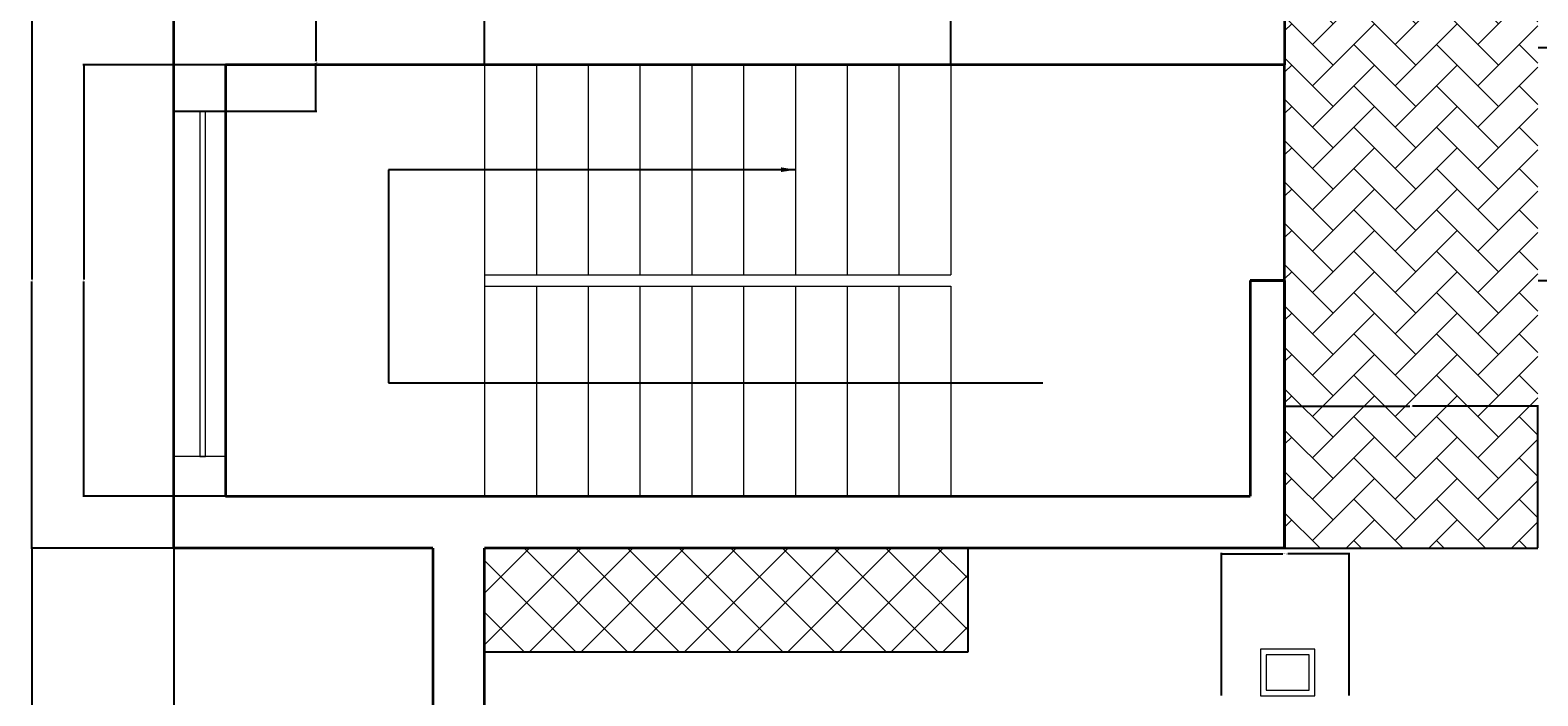
# Model space of a CAD drawing. Units: inches. Extents: x 1315 to 1802, y 1702 to 2202.
# Tile 2 of 4: x 1315 to 1577, y 1906 to 2021. Entities that reach past the tile are written whole.
import ezdxf

# ---------------------------------------------------------------- set-up
doc = ezdxf.new("R2010")
doc.units = ezdxf.units.IN
for name, color, linetype, lineweight in [('A-ANNO-DIMS', 2, 'Continuous', 18), ('A-CASE', 7, 'Continuous', 25), ('A-CASE-PATT', 246, 'Continuous', 13), ('A-FLOR', 7, 'Continuous', 25), ('A-FLOR-PATT', 254, 'Continuous', 13), ('A-FLOR-STRS', 7, 'Continuous', 18), ('A-FURN', 8, 'Continuous', 18), ('A-GLAZ', 4, 'Continuous', 18), ('A-WALL', 7, 'Continuous', 35)]:
    doc.layers.add(name, color=color, linetype=linetype, lineweight=lineweight)
doc.styles.get("Standard").update_dxf_attribs({"font": 'times.ttf'})
doc.dimstyles.new('ISO-25', dxfattribs={"dimtxt": 2.5, "dimasz": 2.5, "dimexe": 1.25, "dimexo": 0.625, "dimtad": 1, "dimdsep": 46, "dimlunit": 3, "dimtxsty": 'Standard', "dimcen": 5, "dimadec": 0, "dimazin": 0, "dimtfac": 1, "dimtmove": 0, "dimatfit": 3, "dimfxl": 1, "dimarcsym": 0})
doc.dimstyles.get("Standard").update_dxf_attribs({"dimtxt": 0.18, "dimasz": 0.18, "dimexe": 0.18, "dimexo": 0.0625, "dimgap": 0.09, "dimtad": 0, "dimtih": 1, "dimtoh": 1, "dimdec": 4, "dimzin": 0, "dimdsep": 46, "dimtxsty": 'Standard', "dimcen": 0.09, "dimadec": 0, "dimazin": 0, "dimtfac": 1, "dimtdec": 4, "dimtofl": 0, "dimtmove": 0, "dimatfit": 3, "dimfxl": 1, "dimtolj": 1, "dimtzin": 0, "dimarcsym": 0})

# ---------------------------------------------------------------- blocks, each defined once
blk = doc.blocks.new('SEFVFT')
for p, q in [((1768.59, 1985.26), (1777.59, 1985.26)), ((1768.59, 1925.26), (1768.59, 1985.26)), ((1768.59, 1985.26), (1773.09, 1985.26)), ((1773.09, 1985.26), (1773.09, 1925.26)), ((1774.09, 1925.26), (1774.09, 1985.26)), ((1777.59, 1985.26), (1777.59, 1925.26)), ((1777.59, 1925.26), (1768.59, 1925.26)), ((1773.09, 1925.26), (1774.09, 1925.26))]:
    blk.add_line(p, q)
blk = doc.blocks.new('CHAIR-DINING-END')
for points in [[(0, 0), (9.48, 0), (9.48, 8.13), (0, 8.13)], [(1, 1), (8.48, 1), (8.48, 7.13), (1, 7.13)]]:
    blk.add_lwpolyline(points, close=True)
blk = doc.blocks.new('*D28')
at = {"layer": 'A-ANNO-DIMS', "color": 0, "lineweight": -2, "transparency": 16777216}
for p, q in [((1339.59, 1931.18), (1339.59, 1702.41)), ((1777.59, 1763.18), (1777.59, 1702.41)), ((1339.77, 1702.59), (1558.31, 1702.59)), ((1777.41, 1702.59), (1558.87, 1702.59))]:
    blk.add_line(p, q, dxfattribs=at)
at = {"layer": 'A-ANNO-DIMS', "color": 0, "transparency": 16777216}
for points in [[(1339.77, 1702.62), (1339.77, 1702.56), (1339.59, 1702.59)], [(1777.41, 1702.62), (1777.41, 1702.56), (1777.59, 1702.59)]]:
    blk.add_solid(points, dxfattribs=at)
at = {"layer": 'Defpoints', "color": 0, "transparency": 16777216}
for p in [(1339.59, 1931.24), (1777.59, 1763.24), (1777.59, 1702.59)]:
    blk.add_point(p, dxfattribs=at)
at = {"layer": 'A-ANNO-DIMS', "color": 0, "transparency": 16777216, "insert": (1558.59, 1702.59), "char_height": 0.18, "attachment_point": 5}
blk.add_mtext('\\A1;438', dxfattribs=at)
blk = doc.blocks.new('*D37')
at = {"layer": 'A-ANNO-DIMS', "color": 0, "lineweight": -2, "transparency": 16777216}
for p, q in [((1339.53, 2024.24), (1314.76, 2024.24)), ((1314.94, 2024.06), (1314.94, 1977.92)), ((1314.94, 1931.42), (1314.94, 1977.56)), ((1339.53, 1931.24), (1314.76, 1931.24))]:
    blk.add_line(p, q, dxfattribs=at)
at = {"layer": 'A-ANNO-DIMS', "color": 0, "transparency": 16777216}
for points in [[(1314.91, 2024.06), (1314.97, 2024.06), (1314.94, 2024.24)], [(1314.91, 1931.42), (1314.97, 1931.42), (1314.94, 1931.24)]]:
    blk.add_solid(points, dxfattribs=at)
at = {"layer": 'Defpoints', "color": 0, "transparency": 16777216}
for p in [(1339.59, 2024.24), (1314.94, 1931.24), (1339.59, 1931.24)]:
    blk.add_point(p, dxfattribs=at)
at = {"layer": 'A-ANNO-DIMS', "color": 0, "transparency": 16777216, "insert": (1314.94, 1977.74), "char_height": 0.18, "attachment_point": 5}
blk.add_mtext('\\A1;93', dxfattribs=at)
blk = doc.blocks.new('*D38')
at = {"layer": 'A-ANNO-DIMS', "color": 0, "lineweight": -2, "transparency": 16777216}
for p, q in [((1339.65, 2024.24), (1364.42, 2024.24)), ((1364.24, 2024.06), (1364.24, 2015.88)), ((1364.24, 2007.33), (1364.24, 2015.51)), ((1339.65, 2007.15), (1364.42, 2007.15))]:
    blk.add_line(p, q, dxfattribs=at)
at = {"layer": 'A-ANNO-DIMS', "color": 0, "transparency": 16777216}
for points in [[(1364.21, 2024.06), (1364.27, 2024.06), (1364.24, 2024.24)], [(1364.21, 2007.33), (1364.27, 2007.33), (1364.24, 2007.15)]]:
    blk.add_solid(points, dxfattribs=at)
at = {"layer": 'Defpoints', "color": 0, "transparency": 16777216}
for p in [(1339.59, 2024.24), (1339.59, 2007.15), (1364.24, 2007.15)]:
    blk.add_point(p, dxfattribs=at)
at = {"layer": 'A-ANNO-DIMS', "color": 0, "transparency": 16777216, "insert": (1364.24, 2015.69), "char_height": 0.18, "attachment_point": 5}
blk.add_mtext('\\A1;17.095', dxfattribs=at)
blk = doc.blocks.new('*D39')
at = {"layer": 'A-ANNO-DIMS', "color": 0, "lineweight": -2, "transparency": 16777216}
for p, q in [((1384.53, 1931.24), (1314.76, 1931.24)), ((1314.94, 1931.06), (1314.94, 1901.56)), ((1314.94, 1871.7), (1314.94, 1901.2)), ((1384.53, 1871.52), (1314.76, 1871.52))]:
    blk.add_line(p, q, dxfattribs=at)
at = {"layer": 'A-ANNO-DIMS', "color": 0, "transparency": 16777216}
for points in [[(1314.91, 1931.06), (1314.97, 1931.06), (1314.94, 1931.24)], [(1314.91, 1871.7), (1314.97, 1871.7), (1314.94, 1871.52)]]:
    blk.add_solid(points, dxfattribs=at)
at = {"layer": 'Defpoints', "color": 0, "transparency": 16777216}
for p in [(1384.59, 1931.24), (1314.94, 1871.52), (1384.59, 1871.52)]:
    blk.add_point(p, dxfattribs=at)
at = {"layer": 'A-ANNO-DIMS', "color": 0, "transparency": 16777216, "insert": (1314.94, 1901.38), "char_height": 0.18, "attachment_point": 5}
blk.add_mtext('\\A1;59.72', dxfattribs=at)
blk = doc.blocks.new('*D49')
at = {"layer": 'A-ANNO-DIMS', "color": 0, "lineweight": -2, "transparency": 16777216}
for p, q in [((1532.59, 1931.3), (1532.59, 1956.07)), ((1532.77, 1955.89), (1554.37, 1955.89)), ((1576.41, 1955.89), (1554.81, 1955.89)), ((1576.59, 1931.3), (1576.59, 1956.07))]:
    blk.add_line(p, q, dxfattribs=at)
at = {"layer": 'A-ANNO-DIMS', "color": 0, "transparency": 16777216}
for points in [[(1532.77, 1955.92), (1532.77, 1955.86), (1532.59, 1955.89)], [(1576.41, 1955.92), (1576.41, 1955.86), (1576.59, 1955.89)]]:
    blk.add_solid(points, dxfattribs=at)
at = {"layer": 'Defpoints', "color": 0, "transparency": 16777216}
for p in [(1576.59, 1955.89), (1532.59, 1931.24), (1576.59, 1931.24)]:
    blk.add_point(p, dxfattribs=at)
at = {"layer": 'A-ANNO-DIMS', "color": 0, "transparency": 16777216, "insert": (1554.59, 1955.89), "char_height": 0.18, "attachment_point": 5}
blk.add_mtext('\\A1;44', dxfattribs=at)
blk = doc.blocks.new('*D50')
at = {"layer": 'A-ANNO-DIMS', "color": 0, "lineweight": -2, "transparency": 16777216}
for p, q in [((1393.59, 2015.3), (1393.59, 2040.07)), ((1393.77, 2039.89), (1433.89, 2039.89)), ((1474.41, 2039.89), (1434.29, 2039.89)), ((1474.59, 2015.3), (1474.59, 2040.07))]:
    blk.add_line(p, q, dxfattribs=at)
at = {"layer": 'A-ANNO-DIMS', "color": 0, "transparency": 16777216}
for points in [[(1393.77, 2039.92), (1393.77, 2039.86), (1393.59, 2039.89)], [(1474.41, 2039.92), (1474.41, 2039.86), (1474.59, 2039.89)]]:
    blk.add_solid(points, dxfattribs=at)
at = {"layer": 'Defpoints', "color": 0, "transparency": 16777216}
for p in [(1474.59, 2039.89), (1393.59, 2015.24), (1474.59, 2015.24)]:
    blk.add_point(p, dxfattribs=at)
at = {"layer": 'A-ANNO-DIMS', "color": 0, "transparency": 16777216, "insert": (1434.09, 2039.89), "char_height": 0.18, "attachment_point": 5}
blk.add_mtext('\\A1;81', dxfattribs=at)
blk = doc.blocks.new('*D51')
at = {"layer": 'A-ANNO-DIMS', "color": 0, "lineweight": -2, "transparency": 16777216}
for p, q in [((1348.53, 2015.24), (1323.76, 2015.24)), ((1323.94, 2015.06), (1323.94, 1977.92)), ((1323.94, 1940.42), (1323.94, 1977.56)), ((1348.53, 1940.24), (1323.76, 1940.24))]:
    blk.add_line(p, q, dxfattribs=at)
at = {"layer": 'A-ANNO-DIMS', "color": 0, "transparency": 16777216}
for points in [[(1323.91, 2015.06), (1323.97, 2015.06), (1323.94, 2015.24)], [(1323.91, 1940.42), (1323.97, 1940.42), (1323.94, 1940.24)]]:
    blk.add_solid(points, dxfattribs=at)
at = {"layer": 'Defpoints', "color": 0, "transparency": 16777216}
for p in [(1323.94, 2015.24), (1348.59, 2015.24), (1348.59, 1940.24)]:
    blk.add_point(p, dxfattribs=at)
at = {"layer": 'A-ANNO-DIMS', "color": 0, "transparency": 16777216, "insert": (1323.94, 1977.74), "char_height": 0.18, "attachment_point": 5}
blk.add_mtext('\\A1;75', dxfattribs=at)
blk = doc.blocks.new('*D52')
at = {"layer": 'A-ANNO-DIMS', "color": 0, "lineweight": -2, "transparency": 16777216}
for p, q in [((1576.65, 2018.24), (1601.42, 2018.24)), ((1601.24, 2018.06), (1601.24, 1998.17)), ((1601.24, 1977.92), (1601.24, 1997.81)), ((1576.65, 1977.74), (1601.42, 1977.74))]:
    blk.add_line(p, q, dxfattribs=at)
at = {"layer": 'A-ANNO-DIMS', "color": 0, "transparency": 16777216}
for points in [[(1601.21, 2018.06), (1601.27, 2018.06), (1601.24, 2018.24)], [(1601.21, 1977.92), (1601.27, 1977.92), (1601.24, 1977.74)]]:
    blk.add_solid(points, dxfattribs=at)
at = {"layer": 'Defpoints', "color": 0, "transparency": 16777216}
for p in [(1576.59, 2018.24), (1576.59, 1977.74), (1601.24, 1977.74)]:
    blk.add_point(p, dxfattribs=at)
at = {"layer": 'A-ANNO-DIMS', "color": 0, "transparency": 16777216, "insert": (1601.24, 1997.99), "char_height": 0.18, "attachment_point": 5}
blk.add_mtext('\\A1;40.5', dxfattribs=at)
blk = doc.blocks.new('*D55')
at = {"layer": 'A-ANNO-DIMS', "color": 0, "lineweight": -2, "transparency": 16777216}
for p, q in [((1521.64, 1905.63), (1521.64, 1930.4)), ((1521.82, 1930.22), (1532.27, 1930.22)), ((1543.62, 1930.22), (1533.17, 1930.22)), ((1543.8, 1905.63), (1543.8, 1930.4))]:
    blk.add_line(p, q, dxfattribs=at)
at = {"layer": 'A-ANNO-DIMS', "color": 0, "transparency": 16777216}
for points in [[(1521.82, 1930.25), (1521.82, 1930.19), (1521.64, 1930.22)], [(1543.62, 1930.25), (1543.62, 1930.19), (1543.8, 1930.22)]]:
    blk.add_solid(points, dxfattribs=at)
at = {"layer": 'Defpoints', "color": 0, "transparency": 16777216}
for p in [(1543.8, 1930.22), (1521.64, 1905.57), (1543.8, 1905.57)]:
    blk.add_point(p, dxfattribs=at)
at = {"layer": 'A-ANNO-DIMS', "color": 0, "transparency": 16777216, "insert": (1532.72, 1930.22), "char_height": 0.18, "attachment_point": 5}
blk.add_mtext('\\A1;22.164', dxfattribs=at)

msp = doc.modelspace()

# ---------------------------------------------------------------- hatches: boundary and pattern name
at = {"layer": 'A-CASE-PATT'}
h = msp.add_hatch(dxfattribs=at)
h.set_pattern_fill('ANSI37', color=256, scale=2)
h.paths.add_polyline_path([(1477.5889, 1931.2411), (1393.5889, 1931.2411), (1393.5889, 1913.2411), (1477.5889, 1913.2411)])
at = {"layer": 'A-FLOR-PATT'}
h = msp.add_hatch(dxfattribs=at)
h.set_pattern_fill('AR-HBONE', color=256, scale=0.05)
h.paths.add_polyline_path([(1576.5889, 2024.2411), (1629.5889, 2024.2411), (1629.5889, 2060.2411), (1629.5889, 2113.2411), (1587.5889, 2113.2411), (1587.5889, 2077.2411), (1532.5889, 2077.2411), (1532.5889, 2015.2411), (1532.5889, 1931.2411), (1576.5889, 1931.2411), (1576.5889, 1940.2411)])
h.paths.add_polyline_path([(1533.7746, 2061.9724), (1533.7746, 2075.958), (1570.2638, 2075.958), (1570.2638, 2061.9724)], flags=16)
edge = h.paths.add_edge_path(flags=0)
edge.add_ellipse((1551.6328, 2068.3646), major_axis=(-10.9397, 0), ratio=0.44313735, start_angle=273.23456, end_angle=623.06073, ccw=False)
edge.add_line((1551.359, 2073.2109), (1551.359, 2073.9173))
edge.add_line((1551.359, 2073.9173), (1552.222, 2073.9173))
edge.add_line((1552.222, 2073.9173), (1552.222, 2073.2053))
h.paths.add_polyline_path([(1551.0754, 2068.4287, -1), (1552.5545, 2068.4287, -1)], flags=0)

# ---------------------------------------------------------------- linework, layer by layer
at = {"layer": 'A-CASE'}
for p, q in [((1393.5889, 1931.2411), (1393.5889, 1913.2411)), ((1477.5889, 1913.2411), (1477.5889, 1931.2411)), ((1393.5889, 1913.2411), (1477.5889, 1913.2411))]:
    msp.add_line(p, q, dxfattribs=at)
at = {"layer": 'A-FLOR'}
msp.add_line((1532.5889, 1931.2411), (1576.5889, 1931.2411), dxfattribs=at)
at = {"layer": 'A-FLOR-STRS'}
for p, q in [((1393.5889, 2015.2411), (1393.5889, 1940.2411)), ((1402.5889, 2015.2411), (1402.5889, 1978.7411)), ((1411.5889, 2015.2411), (1411.5889, 1978.7411)), ((1420.5889, 2015.2411), (1420.5889, 1978.7411)), ((1429.5889, 2015.2411), (1429.5889, 1978.7411)), ((1438.5889, 2015.2411), (1438.5889, 1978.7411)), ((1447.5889, 2015.2411), (1447.5889, 1978.7411)), ((1456.5889, 2015.2411), (1456.5889, 1978.7411)), ((1465.5889, 2015.2411), (1465.5889, 1978.7411)), ((1474.5889, 2015.2411), (1474.5889, 1978.7411)), ((1393.5889, 1978.7411), (1474.5889, 1978.7411)), ((1393.5889, 1976.7411), (1474.5889, 1976.7411)), ((1402.5889, 1976.7411), (1402.5889, 1940.2411)), ((1411.5889, 1976.7411), (1411.5889, 1940.2411)), ((1420.5889, 1976.7411), (1420.5889, 1940.2411)), ((1429.5889, 1976.7411), (1429.5889, 1940.2411)), ((1438.5889, 1976.7411), (1438.5889, 1940.2411)), ((1447.5889, 1976.7411), (1447.5889, 1940.2411)), ((1456.5889, 1976.7411), (1456.5889, 1940.2411)), ((1465.5889, 1976.7411), (1465.5889, 1940.2411)), ((1474.5889, 1976.7411), (1474.5889, 1940.2411))]:
    msp.add_line(p, q, dxfattribs=at)
at = {"layer": 'A-WALL'}
for p, q in [((1532.5889, 2077.2411), (1532.5889, 2015.2411)), ((1339.5889, 1931.2411), (1339.5889, 2024.2411)), ((1532.5889, 2015.2411), (1348.5889, 2015.2411)), ((1348.5889, 2015.2411), (1348.5889, 1940.2411)), ((1532.5889, 1931.2411), (1532.5889, 2015.2411)), ((1526.5889, 1977.7411), (1532.5889, 1977.7411)), ((1532.5889, 1977.7411), (1526.5889, 1977.7411)), ((1526.5889, 1977.7411), (1526.5889, 1940.2411)), ((1532.5889, 1977.7411), (1532.5889, 1931.2411)), ((1348.5889, 1940.2411), (1526.5889, 1940.2411)), ((1348.5889, 1931.2411), (1339.5889, 1931.2411)), ((1384.5889, 1931.2411), (1348.5889, 1931.2411)), ((1384.5889, 1931.2411), (1384.5889, 1790.2411)), ((1532.5889, 1931.2411), (1393.5889, 1931.2411)), ((1393.5889, 1799.2411), (1393.5889, 1931.2411))]:
    msp.add_line(p, q, dxfattribs=at)

# ---------------------------------------------------------------- block references
at = {"layer": 'A-FURN'}
msp.add_blockref('CHAIR-DINING-END', (1528.381, 1905.568), dxfattribs=at)
at = {"layer": 'A-GLAZ'}
msp.add_blockref('SEFVFT', (-429, 21.8903), dxfattribs=at)

# ---------------------------------------------------------------- dimensions: what is measured, and where the dimension line sits
at = {"layer": 'A-ANNO-DIMS'}
for base, p1, p2, override, picture, middle in [((1474.5889, 2039.8911), (1393.5889, 2015.2411), (1474.5889, 2015.2411), {"dimdec": 0, "dimlfac": 1, "dimrnd": 0, "dimzin": 0, "dimdsep": 46, "dimlunit": 2}, '*D50', (1434.0889, 2039.8911)), ((1576.5889, 1955.8911), (1532.5889, 1931.2411), (1576.5889, 1931.2411), {"dimdec": 0, "dimlfac": 1, "dimrnd": 0, "dimzin": 0, "dimdsep": 46, "dimlunit": 2}, '*D49', (1554.5889, 1955.8911)), ((1777.5889, 1702.5911), (1339.5889, 1931.2411), (1777.5889, 1763.2411), {"dimdec": 0, "dimlfac": 1, "dimrnd": 0, "dimzin": 0, "dimdsep": 46, "dimlunit": 2}, '*D28', (1558.5889, 1702.5911)), ((1543.7995, 1930.2183), (1521.6357, 1905.5683), (1543.7995, 1905.5683), {"dimdec": 3, "dimlfac": 1, "dimrnd": 0, "dimzin": 0, "dimdsep": 46, "dimlunit": 2}, '*D55', (1532.7176, 1930.2183))]:
    dim = msp.add_linear_dim(base=base, p1=p1, p2=p2, dimstyle='Standard', override=override, dxfattribs=at)
    dim.commit()
    dim.dimension.update_dxf_attribs({"geometry": picture, "text_midpoint": middle})
for base, p1, p2, angle, override, picture, middle in [((1314.9389, 1931.2411), (1339.5889, 2024.2411), (1339.5889, 1931.2411), 90, {"dimdec": 0, "dimlfac": 1, "dimrnd": 0, "dimzin": 0, "dimdsep": 46, "dimlunit": 2}, '*D37', (1314.9389, 1977.7411)), ((1364.2389, 2007.1462), (1339.5889, 2024.2411), (1339.5889, 2007.1462), 270, {"dimdec": 3, "dimlfac": 1, "dimrnd": 0, "dimzin": 0, "dimdsep": 46, "dimlunit": 2}, '*D38', (1364.2389, 2015.6937)), ((1601.2389, 1977.7411), (1576.5889, 2018.2411), (1576.5889, 1977.7411), 270, {"dimdec": 1, "dimlfac": 1, "dimrnd": 0, "dimzin": 0, "dimdsep": 46, "dimlunit": 2}, '*D52', (1601.2389, 1997.9911)), ((1323.9389, 2015.2411), (1348.5889, 1940.2411), (1348.5889, 2015.2411), 90, {"dimdec": 0, "dimlfac": 1, "dimrnd": 0, "dimzin": 0, "dimdsep": 46, "dimlunit": 2}, '*D51', (1323.9389, 1977.7411)), ((1314.9389, 1871.5173), (1384.5889, 1931.2411), (1384.5889, 1871.5173), 90, {"dimdec": 2, "dimlfac": 1, "dimrnd": 0, "dimzin": 0, "dimdsep": 46, "dimlunit": 2}, '*D39', (1314.9389, 1901.3792))]:
    dim = msp.add_linear_dim(base=base, p1=p1, p2=p2, angle=angle, dimstyle='Standard', override=override, dxfattribs=at)
    dim.commit()
    dim.dimension.update_dxf_attribs({"geometry": picture, "text_midpoint": middle})

# ---------------------------------------------------------------- leaders
at = {"layer": 'A-FLOR-STRS'}
msp.add_leader([(1447.5889, 1996.9911), (1376.9014, 1996.9911), (1376.9014, 1959.9372), (1490.601, 1959.9372)], dimstyle='ISO-25', dxfattribs=at)

doc.saveas('drawing.dxf')
